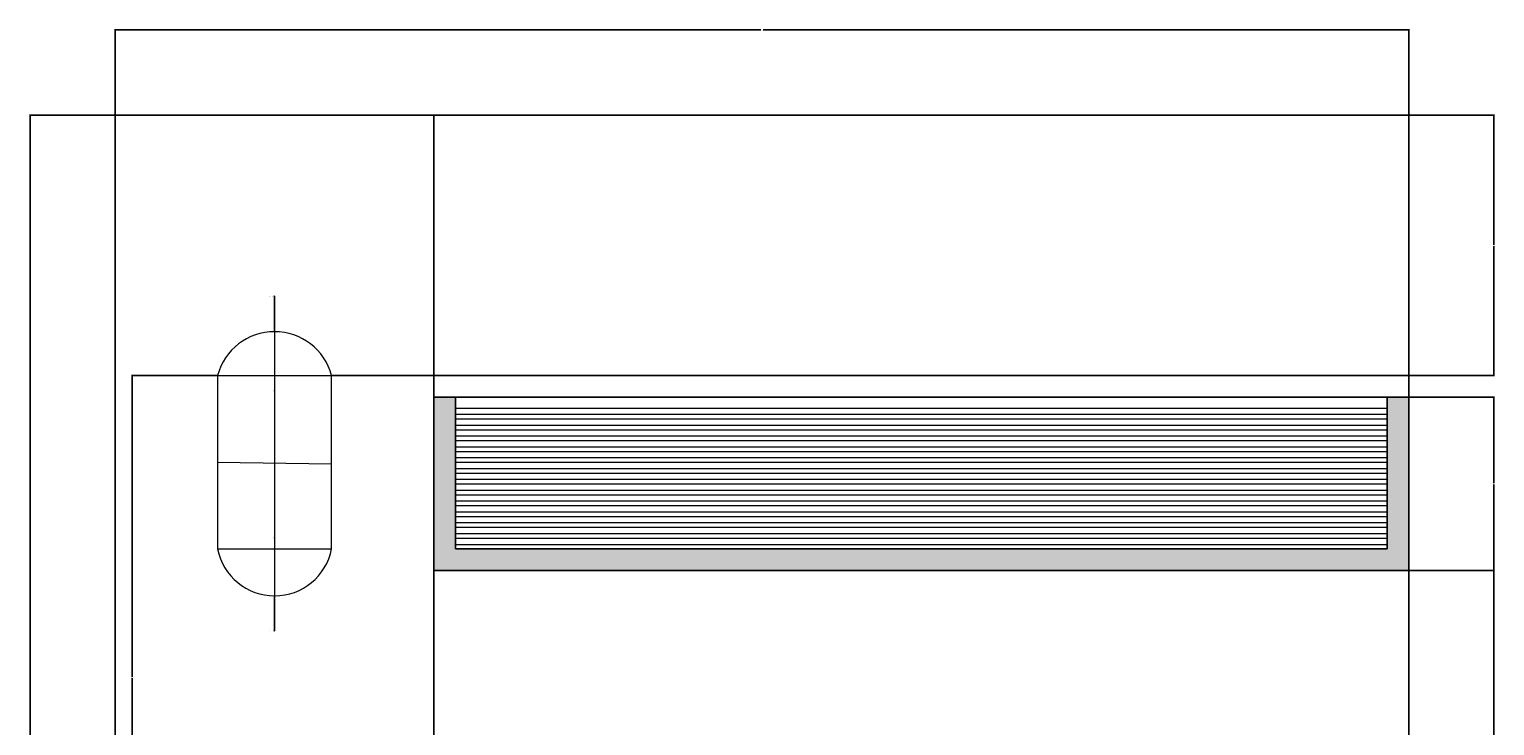
# Model space of a CAD drawing. Units: inches. Extents: x 3504 to 4623, y 2365 to 3357.
# Tile 3 of 5: x 3504 to 3909, y 3164 to 3357. Entities that reach past the tile are written whole.
import ezdxf

# ---------------------------------------------------------------- set-up
doc = ezdxf.new("R2010")
doc.units = ezdxf.units.IN
for name, color, linetype, lineweight in [('A-ANNO-DIMS', 2, 'Continuous', 18), ('A-ELEV', 7, 'Continuous', 25), ('A-ELEV-PATT', 7, 'Continuous', 13), ('A-FLOR-HRAL', 7, 'Continuous', 25), ('A-FLOR-HRAL-PATT', 252, 'Continuous', 13), ('A-GLAZ', 4, 'Continuous', 18)]:
    doc.layers.add(name, color=color, linetype=linetype, lineweight=lineweight)
doc.styles.get("Standard").update_dxf_attribs({"font": 'arial.ttf'})
doc.dimstyles.get("Standard").update_dxf_attribs({"dimtxt": 0.18, "dimasz": 0.18, "dimexe": 0.18, "dimexo": 0.0625, "dimgap": 0.09, "dimtad": 0, "dimtih": 1, "dimtoh": 1, "dimdec": 4, "dimzin": 0, "dimdsep": 46, "dimtxsty": 'Standard', "dimcen": 0.09, "dimadec": 0, "dimazin": 0, "dimtfac": 1, "dimtdec": 4, "dimtofl": 0, "dimtmove": 0, "dimatfit": 3, "dimfxl": 1, "dimtolj": 1, "dimtzin": 0, "dimarcsym": 0})

# ---------------------------------------------------------------- blocks, each defined once
blk = doc.blocks.new('WIN-ARCH-END-ELEV')
for p, q in [((15.78, 73.08), (15.78, 0)), ((0, 60.97), (31.56, 60.97)), ((0, 60.97), (0, 12.97)), ((31.56, 12.97), (31.56, 60.97)), ((0, 36.97), (31.56, 36.54)), ((0, 12.97), (31.56, 12.97)), ((0, 12.97), (31.56, 12.97))]:
    blk.add_line(p, q)
for centre, radius, start, end in [((15.78, 56.75), 16.33, 14.9627, 165.0373), ((15.78, 16.08), 16.08, 191.1699, 348.8301)]:
    blk.add_arc(centre, radius, start, end)
blk = doc.blocks.new('*D47')
at = {"layer": 'A-ANNO-DIMS', "color": 0, "lineweight": -2, "transparency": 16777216}
for p, q in [((3527.5, 3333.05), (3527.5, 3356.76)), ((3527.68, 3356.58), (3706.21, 3356.58)), ((3885.32, 3356.58), (3706.79, 3356.58)), ((3885.5, 3255.05), (3885.5, 3356.76))]:
    blk.add_line(p, q, dxfattribs=at)
at = {"layer": 'A-ANNO-DIMS', "color": 0, "transparency": 16777216}
for points in [[(3527.68, 3356.61), (3527.68, 3356.55), (3527.5, 3356.58)], [(3885.32, 3356.61), (3885.32, 3356.55), (3885.5, 3356.58)]]:
    blk.add_solid(points, dxfattribs=at)
at = {"layer": 'Defpoints', "color": 0, "transparency": 16777216}
for p in [(3885.5, 3356.58), (3527.5, 3332.98), (3885.5, 3254.98)]:
    blk.add_point(p, dxfattribs=at)
at = {"layer": 'A-ANNO-DIMS', "color": 0, "transparency": 16777216, "insert": (3706.5, 3356.58), "char_height": 0.18, "attachment_point": 5}
blk.add_mtext('\\A1;358', dxfattribs=at)
blk = doc.blocks.new('*D59')
at = {"layer": 'A-ANNO-DIMS', "color": 0, "lineweight": -2, "transparency": 16777216}
for p, q in [((3885.56, 3206.98), (3909.28, 3206.98)), ((3909.1, 3206.8), (3909.1, 3126.17)), ((3909.1, 3045.16), (3909.1, 3125.8)), ((3885.56, 3044.98), (3909.28, 3044.98))]:
    blk.add_line(p, q, dxfattribs=at)
at = {"layer": 'A-ANNO-DIMS', "color": 0, "transparency": 16777216}
for points in [[(3909.07, 3206.8), (3909.13, 3206.8), (3909.1, 3206.98)], [(3909.07, 3045.16), (3909.13, 3045.16), (3909.1, 3044.98)]]:
    blk.add_solid(points, dxfattribs=at)
at = {"layer": 'Defpoints', "color": 0, "transparency": 16777216}
for p in [(3885.5, 3206.98), (3909.1, 3206.98), (3885.5, 3044.98)]:
    blk.add_point(p, dxfattribs=at)
at = {"layer": 'A-ANNO-DIMS', "color": 0, "transparency": 16777216, "insert": (3909.1, 3125.98), "char_height": 0.18, "attachment_point": 5}
blk.add_mtext('\\A1;162', dxfattribs=at)
blk = doc.blocks.new('*D60')
at = {"layer": 'A-ANNO-DIMS', "color": 0, "lineweight": -2, "transparency": 16777216}
for p, q in [((3885.56, 3254.98), (3909.28, 3254.98)), ((3909.1, 3254.8), (3909.1, 3231.17)), ((3909.1, 3207.16), (3909.1, 3230.8)), ((3885.56, 3206.98), (3909.28, 3206.98))]:
    blk.add_line(p, q, dxfattribs=at)
at = {"layer": 'A-ANNO-DIMS', "color": 0, "transparency": 16777216}
for points in [[(3909.07, 3254.8), (3909.13, 3254.8), (3909.1, 3254.98)], [(3909.07, 3207.16), (3909.13, 3207.16), (3909.1, 3206.98)]]:
    blk.add_solid(points, dxfattribs=at)
at = {"layer": 'Defpoints', "color": 0, "transparency": 16777216}
for p in [(3885.5, 3254.98), (3909.1, 3254.98), (3885.5, 3206.98)]:
    blk.add_point(p, dxfattribs=at)
at = {"layer": 'A-ANNO-DIMS', "color": 0, "transparency": 16777216, "insert": (3909.1, 3230.98), "char_height": 0.18, "attachment_point": 5}
blk.add_mtext('\\A1;48', dxfattribs=at)
blk = doc.blocks.new('*D61')
at = {"layer": 'A-ANNO-DIMS', "color": 0, "lineweight": -2, "transparency": 16777216}
for p, q in [((3555.74, 3260.98), (3532.02, 3260.98)), ((3532.2, 3260.8), (3532.2, 3177.56)), ((3532.2, 3093.96), (3532.2, 3177.2)), ((3555.74, 3093.78), (3532.02, 3093.78))]:
    blk.add_line(p, q, dxfattribs=at)
at = {"layer": 'A-ANNO-DIMS', "color": 0, "transparency": 16777216}
for points in [[(3532.17, 3260.8), (3532.23, 3260.8), (3532.2, 3260.98)], [(3532.17, 3093.96), (3532.23, 3093.96), (3532.2, 3093.78)]]:
    blk.add_solid(points, dxfattribs=at)
at = {"layer": 'Defpoints', "color": 0, "transparency": 16777216}
for p in [(3532.2, 3260.98), (3555.8, 3260.98), (3555.8, 3093.78)]:
    blk.add_point(p, dxfattribs=at)
at = {"layer": 'A-ANNO-DIMS', "color": 0, "transparency": 16777216, "insert": (3532.2, 3177.38), "char_height": 0.18, "attachment_point": 5}
blk.add_mtext('\\A1;167.2', dxfattribs=at)
blk = doc.blocks.new('*D62')
at = {"layer": 'A-ANNO-DIMS', "color": 0, "lineweight": -2, "transparency": 16777216}
for p, q in [((3615.73, 3332.98), (3909.28, 3332.98)), ((3909.1, 3332.8), (3909.1, 3297.16)), ((3909.1, 3261.16), (3909.1, 3296.8)), ((3587.42, 3260.98), (3909.28, 3260.98))]:
    blk.add_line(p, q, dxfattribs=at)
at = {"layer": 'A-ANNO-DIMS', "color": 0, "transparency": 16777216}
for points in [[(3909.07, 3332.8), (3909.13, 3332.8), (3909.1, 3332.98)], [(3909.07, 3261.16), (3909.13, 3261.16), (3909.1, 3260.98)]]:
    blk.add_solid(points, dxfattribs=at)
at = {"layer": 'Defpoints', "color": 0, "transparency": 16777216}
for p in [(3615.67, 3332.98), (3909.1, 3332.98), (3587.36, 3260.98)]:
    blk.add_point(p, dxfattribs=at)
at = {"layer": 'A-ANNO-DIMS', "color": 0, "transparency": 16777216, "insert": (3909.1, 3296.98), "char_height": 0.18, "attachment_point": 5}
blk.add_mtext('\\A1;72', dxfattribs=at)
blk = doc.blocks.new('*D63')
at = {"layer": 'A-ANNO-DIMS', "color": 0, "lineweight": -2, "transparency": 16777216}
for p, q in [((3527.43, 3332.98), (3503.72, 3332.98)), ((3503.9, 3332.8), (3503.9, 3099.17)), ((3503.9, 2865.16), (3503.9, 3098.8)), ((3527.43, 2864.98), (3503.72, 2864.98))]:
    blk.add_line(p, q, dxfattribs=at)
at = {"layer": 'A-ANNO-DIMS', "color": 0, "transparency": 16777216}
for points in [[(3503.87, 3332.8), (3503.93, 3332.8), (3503.9, 3332.98)], [(3503.87, 2865.16), (3503.93, 2865.16), (3503.9, 2864.98)]]:
    blk.add_solid(points, dxfattribs=at)
at = {"layer": 'Defpoints', "color": 0, "transparency": 16777216}
for p in [(3503.9, 3332.98), (3527.5, 3332.98), (3527.5, 2864.98)]:
    blk.add_point(p, dxfattribs=at)
at = {"layer": 'A-ANNO-DIMS', "color": 0, "transparency": 16777216, "insert": (3503.9, 3098.98), "char_height": 0.18, "attachment_point": 5}
blk.add_mtext('\\A1;468', dxfattribs=at)
blk = doc.blocks.new('*D76')
at = {"layer": 'A-ANNO-DIMS', "color": 0, "lineweight": -2, "transparency": 16777216}
for p, q in [((3571.4, 3282.9), (3571.58, 3282.9)), ((3571.58, 3282.9), (3571.58, 3273.28)), ((3571.49, 3256.77), (3571.67, 3256.77)), ((3571.58, 3256.68), (3571.58, 3256.86))]:
    blk.add_line(p, q, dxfattribs=at)
at = {"layer": 'A-ANNO-DIMS', "color": 0, "transparency": 16777216}
blk.add_solid([(3571.61, 3273.28), (3571.55, 3273.28), (3571.58, 3273.1)], dxfattribs=at)
at = {"layer": 'Defpoints', "color": 0, "transparency": 16777216}
for p in [(3571.58, 3273.1), (3571.58, 3256.77)]:
    blk.add_point(p, dxfattribs=at)
at = {"layer": 'A-ANNO-DIMS', "color": 0, "transparency": 16777216, "insert": (3570.66, 3282.9), "char_height": 0.18, "attachment_point": 5}
blk.add_mtext('\\A1;2X R16.333', dxfattribs=at)
blk = doc.blocks.new('*D77')
at = {"layer": 'A-ANNO-DIMS', "color": 0, "lineweight": -2, "transparency": 16777216}
for p, q in [((3571.49, 3216.1), (3571.67, 3216.1)), ((3571.58, 3216.01), (3571.58, 3216.19)), ((3571.58, 3190.37), (3571.58, 3199.84)), ((3571.4, 3190.37), (3571.58, 3190.37))]:
    blk.add_line(p, q, dxfattribs=at)
at = {"layer": 'A-ANNO-DIMS', "color": 0, "transparency": 16777216}
blk.add_solid([(3571.55, 3199.84), (3571.61, 3199.84), (3571.58, 3200.02)], dxfattribs=at)
at = {"layer": 'Defpoints', "color": 0, "transparency": 16777216}
for p in [(3571.58, 3216.1), (3571.58, 3200.02)]:
    blk.add_point(p, dxfattribs=at)
at = {"layer": 'A-ANNO-DIMS', "color": 0, "transparency": 16777216, "insert": (3570.66, 3190.37), "char_height": 0.18, "attachment_point": 5}
blk.add_mtext('\\A1;2X R16.084', dxfattribs=at)

msp = doc.modelspace()

# ---------------------------------------------------------------- hatches: boundary and pattern name
at = {"layer": 'A-ELEV-PATT'}
h = msp.add_hatch(color=256, dxfattribs=at)
h.dxf.hatch_style = 1
h.paths.add_polyline_path([(3885.4963, 3254.9837), (3879.4963, 3254.9837), (3879.4963, 3212.9837), (3621.6665, 3212.9837), (3621.6665, 3254.9837), (3615.6665, 3254.9837), (3615.6665, 3206.9837), (3885.4963, 3206.9837)])
at = {"layer": 'A-FLOR-HRAL-PATT'}
h = msp.add_hatch(dxfattribs=at)
h.set_pattern_fill('ANSI31', color=256, scale=0.944877, angle=-45, style=0)
h.paths.add_polyline_path([(3621.6665, 3212.9937), (3879.4963, 3212.9937), (3879.4963, 3254.9737), (3621.6665, 3254.9737)])
h = msp.add_hatch(dxfattribs=at)
h.set_pattern_fill('ANSI31', color=256, scale=0.945252, angle=-45, style=0)
h.paths.add_polyline_path([(3621.6665, 3212.9837), (3879.4963, 3212.9837), (3879.4963, 3251.764), (3621.6665, 3251.764)])

# ---------------------------------------------------------------- linework, layer by layer
at = {"layer": 'A-ELEV'}
for p, q in [((3527.4963, 3332.9837), (3615.6665, 3332.9837)), ((3527.4963, 2864.9837), (3527.4963, 3332.9837)), ((3615.6665, 2888.9837), (3615.6665, 3332.9837)), ((3885.4963, 2864.9837), (3885.4963, 3254.9837))]:
    msp.add_line(p, q, dxfattribs=at)
at = {"layer": 'A-FLOR-HRAL'}
for p, q in [((3615.6665, 3254.9837), (3885.4963, 3254.9837)), ((3621.6665, 3212.9837), (3621.6665, 3254.9837)), ((3621.6665, 3254.9837), (3879.4963, 3254.9837)), ((3879.4963, 3212.9837), (3879.4963, 3254.9837)), ((3621.6665, 3212.9837), (3879.4963, 3212.9837)), ((3615.6665, 3206.9837), (3885.4963, 3206.9837))]:
    msp.add_line(p, q, dxfattribs=at)

# ---------------------------------------------------------------- block references
at = {"layer": 'A-GLAZ'}
msp.add_blockref('WIN-ARCH-END-ELEV', (3555.8023, 3200.0157), dxfattribs=at)

# ---------------------------------------------------------------- dimensions: what is measured, and where the dimension line sits
at = {"layer": 'A-ANNO-DIMS'}
dim = msp.add_linear_dim(base=(3885.4963, 3356.5837), p1=(3527.4963, 3332.9837), p2=(3885.4963, 3254.9837), dimstyle='Standard', override={"dimdec": 0, "dimlfac": 1, "dimrnd": 0, "dimzin": 0, "dimdsep": 46, "dimlunit": 2}, dxfattribs=at)
dim.commit()
dim.dimension.update_dxf_attribs({"geometry": '*D47', "text_midpoint": (3706.4963, 3356.5837)})
for base, p1, p2, override, picture, middle in [((3503.8963, 3332.9837), (3527.4963, 2864.9837), (3527.4963, 3332.9837), {"dimdec": 0, "dimlfac": 1, "dimrnd": 0, "dimzin": 0, "dimdsep": 46, "dimlunit": 2}, '*D63', (3503.8963, 3098.9837)), ((3909.0963, 3332.9837), (3587.3605, 3260.9837), (3615.6665, 3332.9837), {"dimdec": 0, "dimlfac": 1, "dimrnd": 0, "dimzin": 0, "dimdsep": 46, "dimlunit": 2}, '*D62', (3909.0963, 3296.9837)), ((3532.2023, 3260.9837), (3555.8023, 3093.7806), (3555.8023, 3260.9837), {"dimdec": 1, "dimlfac": 1, "dimrnd": 0, "dimzin": 0, "dimdsep": 46, "dimlunit": 2}, '*D61', (3532.2023, 3177.3822)), ((3909.0963, 3254.9837), (3885.4963, 3206.9837), (3885.4963, 3254.9837), {"dimdec": 0, "dimlfac": 1, "dimrnd": 0, "dimzin": 0, "dimdsep": 46, "dimlunit": 2}, '*D60', (3909.0963, 3230.9837)), ((3909.0963, 3206.9837), (3885.4963, 3044.9837), (3885.4963, 3206.9837), {"dimdec": 0, "dimlfac": 1, "dimrnd": 0, "dimzin": 0, "dimdsep": 46, "dimlunit": 2}, '*D59', (3909.0963, 3125.9837))]:
    dim = msp.add_linear_dim(base=base, p1=p1, p2=p2, angle=90, dimstyle='Standard', override=override, dxfattribs=at)
    dim.commit()
    dim.dimension.update_dxf_attribs({"geometry": picture, "text_midpoint": middle})
for center, mpoint, picture, middle in [((3571.5814, 3256.7667), (3571.581, 3273.0996), '*D76', (3570.6561, 3282.8993)), ((3571.5814, 3216.0994), (3571.581, 3200.0157), '*D77', (3570.6565, 3190.3654))]:
    dim = msp.add_radius_dim(center=center, mpoint=mpoint, text='2X <>', dimstyle='Standard', override={"dimdec": 3, "dimlfac": 1, "dimrnd": 0, "dimzin": 0, "dimdsep": 46, "dimlunit": 2}, dxfattribs=at)
    dim.commit()
    dim.dimension.update_dxf_attribs({"geometry": picture, "text_midpoint": middle, "dimtype": 164})

doc.saveas('drawing.dxf')
